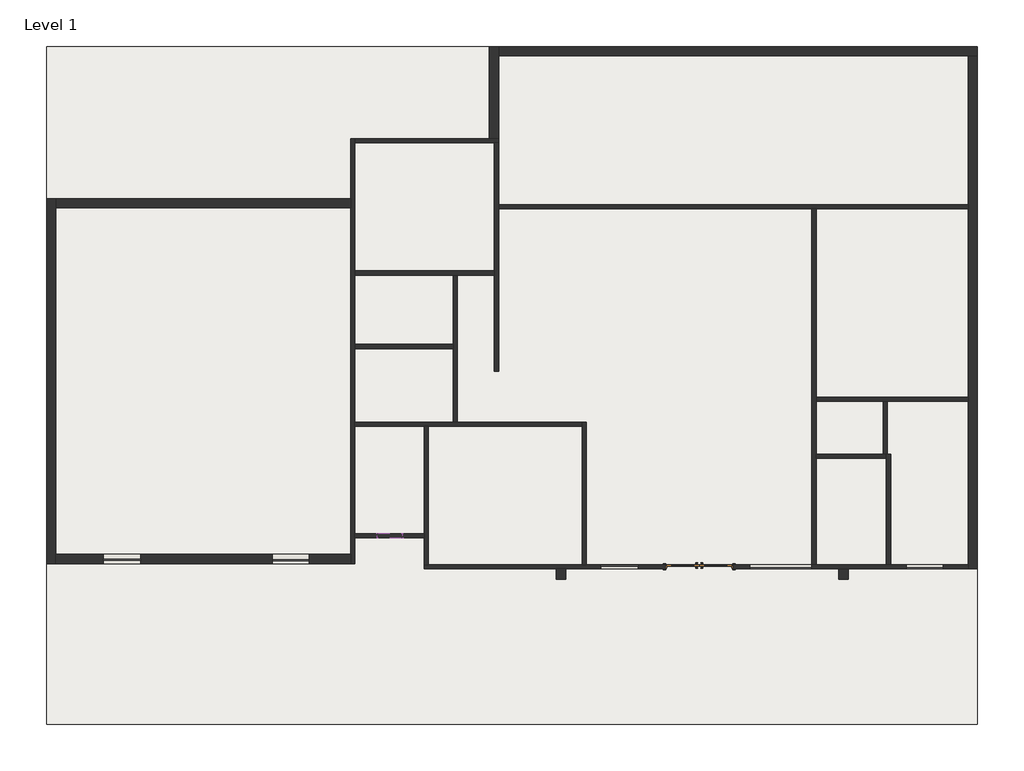
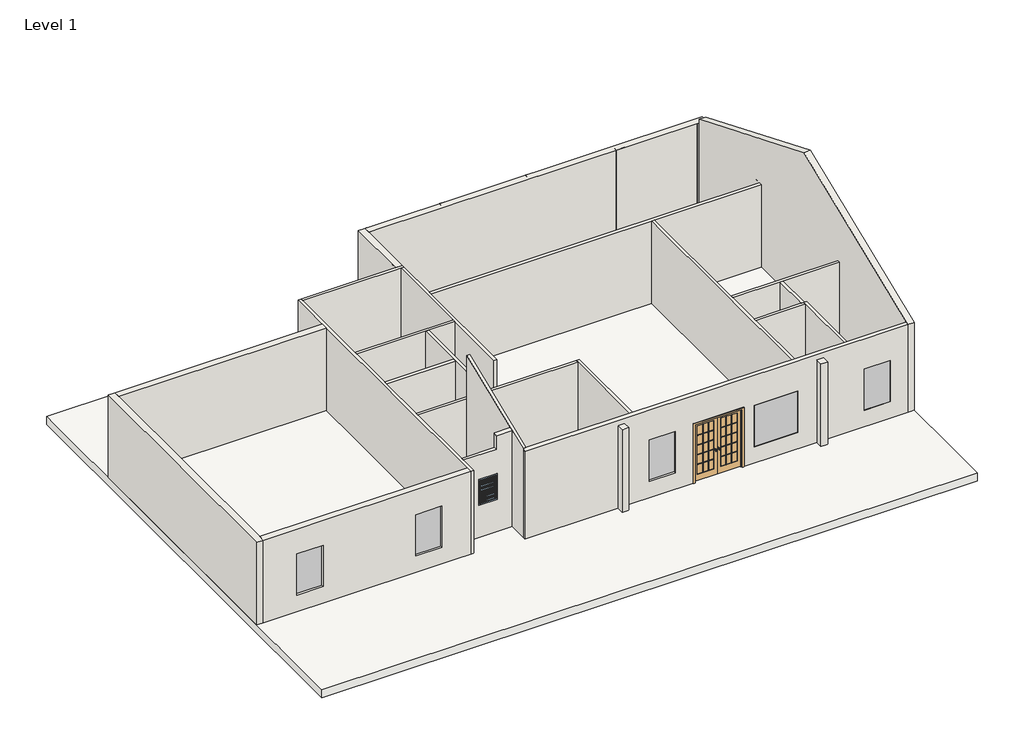
# One storey: 25 walls, 7 columns, 5 plates, 1 door, 1 slab, 1 window.
"""IFC4 building model written with IfcOpenShell, lengths in millimetres."""

from ifc_helpers import new_model, si_unit, frame, origin, origin_with_axes, place, context, project, spatial, polyline, outline, extrude, faceted_brep, transform, mapped, element, save
from components import door_09c896ac, system_panel_glazed_cdc09dc4, system_panel_glazed_afe70ed6, window_d9a389d2

model = new_model("IFC4")

# Units and contexts
model_context = context("Model", 3, world=origin())
ifc_project = project(units=[si_unit("LENGTHUNIT", "METRE", prefix="MILLI")], contexts=[model_context])

# Site, building, storey
site = spatial("IfcSite", under=ifc_project)
building = spatial("IfcBuilding", under=site)
storey = spatial("IfcBuildingStorey", under=building, Name="Level 1", Elevation=0.0)

# Columns
placement = place(None, origin())
element("IfcColumn", 1, ObjectType="Rectangular Column : 9\" x 12\"", at=placement, inside=storey, context=model_context, shape_type="SweptSolid", body=[
    extrude(outline(polyline([(-2253.6765363, 15600.9899709), (-2253.6765363, 15372.3899709), (-2329.8765363, 15372.3899709), (-2329.8765363, 15600.9899709), (-2253.6765363, 15600.9899709)])), origin_with_axes(), (0.0, 0.0, 1.0), 3048.0),
])
element("IfcColumn", 2, ObjectType="Rectangular Column : 9\" x 12\"", at=placement, inside=storey, context=model_context, shape_type="Brep", body=[
    faceted_brep([(9430.3234637, 15600.9899709, 0.0), (9430.3234637, 15372.3899709, 0.0), (9201.7234637, 15372.3899709, 0.0), (9125.5234637, 15372.3899709, 0.0), (9125.5234637, 15600.9899709, 0.0), (9430.3234637, 15600.9899709, 3048.0), (9430.3234637, 15372.3899709, 3048.0), (9125.5234637, 15372.3899709, 3048.0), (9125.5234637, 15600.9899709, 3048.0)], [[[0, 1, 2, 3, 4]], [[5, 6, 1, 0]], [[6, 7, 3, 2, 1]], [[7, 8, 4, 3]], [[8, 5, 0, 4]], [[5, 8, 7, 6]]]),
])
element("IfcColumn", 3, ObjectType="Rectangular Column : 9\" x 12\"", at=placement, inside=storey, context=model_context, shape_type="SweptSolid", body=[
    extrude(outline(polyline([(565.7234637, 15600.9899709), (565.7234637, 15372.3899709), (260.9234637, 15372.3899709), (260.9234637, 15600.9899709), (565.7234637, 15600.9899709)])), origin_with_axes(), (0.0, 0.0, 1.0), 3048.0),
])
element("IfcColumn", 4, ObjectType="Rectangular Column : 9\" x 12\"", at=placement, inside=storey, context=model_context, shape_type="SweptSolid", body=[
    extrude(outline(polyline([(3562.9234637, 15600.9899709), (3562.9234637, 15372.3899709), (3258.1234637, 15372.3899709), (3258.1234637, 15600.9899709), (3562.9234637, 15600.9899709)])), origin_with_axes(), (0.0, 0.0, 1.0), 3048.0),
])
element("IfcColumn", 5, ObjectType="Rectangular Column : 9\" x 12\"", at=placement, inside=storey, context=model_context, shape_type="SweptSolid", body=[
    extrude(outline(polyline([(6610.9234637, 15600.9899709), (6610.9234637, 15372.3899709), (6306.1234637, 15372.3899709), (6306.1234637, 15600.9899709), (6610.9234637, 15600.9899709)])), origin_with_axes(), (0.0, 0.0, 1.0), 3048.0),
])
element("IfcColumn", 6, ObjectType="Rectangular Column : 9\" x 12\"", at=placement, inside=storey, context=model_context, shape_type="SweptSolid", body=[
    extrude(outline(polyline([(-2558.4765363, 13543.5899709), (-2329.8765363, 13543.5899709), (-2329.8765363, 13340.3899709), (-2558.4765363, 13340.3899709), (-2558.4765363, 13543.5899709)])), origin_with_axes(), (0.0, 0.0, 1.0), 3048.0),
])
element("IfcColumn", 7, ObjectType="Rectangular Column : 9\" x 12\"", at=placement, inside=storey, context=model_context, shape_type="Brep", body=[
    faceted_brep([(9201.7234637, 11917.9899709, 0.0), (9430.3234637, 11917.9899709, 0.0), (9430.3234637, 11613.1899709, 0.0), (9201.7234637, 11613.1899709, 0.0), (9201.7234637, 11714.7899709, 0.0), (9201.7234637, 11917.9899709, 3048.0), (9430.3234637, 11917.9899709, 3048.0), (9430.3234637, 11613.1899709, 3048.0), (9201.7234637, 11613.1899709, 3048.0), (9201.7234637, 11714.7899709, 3048.0)], [[[0, 1, 2, 3, 4]], [[5, 6, 1, 0]], [[6, 7, 2, 1]], [[7, 8, 3, 2]], [[8, 9, 5, 0, 4, 3]], [[5, 9, 8, 7, 6]]]),
])

# Door
door_shape = door_09c896ac(model_context)
element("IfcDoor", 8, ObjectType="Door-Interior-Double-Full Glass-Wood : 64\" x 84\"", at=placement, inside=storey, context=model_context, shape_type="MappedRepresentation", body=[
    mapped(door_shape, transform((2597.7234637, 2827.9649709, 0.0), x_axis=(1.0, 0.0, 0.0), y_axis=(0.0, 1.0, 0.0), z_axis=(0.0, 0.0, 1.0))),
])

# Plates
system_panel_glazed_shape = system_panel_glazed_cdc09dc4(model_context)
element("IfcPlate", 9, ObjectType="System Panel : Glazed", at=placement, inside=storey, context=model_context, shape_type="MappedRepresentation", body=[
    mapped(system_panel_glazed_shape, transform((641.9234637, 2824.7899709, 609.6), x_axis=(1.0, 0.0, 0.0), y_axis=(0.0, 1.0, 0.0), z_axis=(0.0, 0.0, 1.0))),
])
element("IfcPlate", 10, ObjectType="System Panel : Glazed", at=placement, inside=storey, context=model_context, shape_type="MappedRepresentation", body=[
    mapped(system_panel_glazed_shape, transform((8134.9234637, 2824.7899709, 609.6), x_axis=(-1.0, 0.0, 0.0), y_axis=(0.0, -1.0, 0.0), z_axis=(0.0, 0.0, 1.0))),
])
element("IfcPlate", 11, ObjectType="System Panel : Glazed", at=placement, inside=storey, context=model_context, shape_type="MappedRepresentation", body=[
    mapped(system_panel_glazed_shape, transform((-7435.2765363, 3015.2899709, 609.6), x_axis=(-1.0, 0.0, 0.0), y_axis=(0.0, -1.0, 0.0), z_axis=(0.0, 0.0, 1.0))),
])
element("IfcPlate", 12, ObjectType="System Panel : Glazed", at=placement, inside=storey, context=model_context, shape_type="MappedRepresentation", body=[
    mapped(system_panel_glazed_shape, transform((-11575.4765363, 2964.4899709, 609.6), x_axis=(1.0, 0.0, 0.0), y_axis=(0.0, 1.0, 0.0), z_axis=(0.0, 0.0, 1.0))),
])
system_panel_glazed_2_shape = system_panel_glazed_afe70ed6(model_context)
element("IfcPlate", 13, ObjectType="System Panel : Glazed", at=placement, inside=storey, context=model_context, shape_type="MappedRepresentation", body=[
    mapped(system_panel_glazed_2_shape, transform((4604.3234637, 2824.7899709, 609.6), x_axis=(-1.0, 0.0, 0.0), y_axis=(0.0, -1.0, 0.0), z_axis=(0.0, 0.0, 1.0))),
])

# Slab
element("IfcSlab", 14, ObjectType="Generic - 12\"", at=placement, inside=storey, context=model_context, shape_type="SweptSolid", body=[
    extrude(outline(polyline([(-13429.6765363, 15600.9899709), (9430.3234637, 15600.9899709), (9430.3234637, -1037.5706845), (-13429.6765363, -1037.5706845), (-13429.6765363, 15600.9899709)])), frame((0.0, 0.0, -304.8), z_axis=(0.0, 0.0, 1.0), x_axis=(1.0, 0.0, 0.0)), (0.0, 0.0, 1.0), 304.8),
])

# Walls
element("IfcWall", 15, ObjectType="4\" wall", at=placement, inside=storey, context=model_context, shape_type="Brep", body=[
    faceted_brep([(-2329.8765363, 11613.1899709, 0.0), (5366.3234637, 11613.1899709, 0.0), (5467.9234637, 11613.1899709, 0.0), (9201.7234637, 11613.1899709, 0.0), (9201.7234637, 11613.1899709, 3048.0), (5467.9234637, 11613.1899709, 3048.0), (5366.3234637, 11613.1899709, 3048.0), (-2329.8765363, 11613.1899709, 3048.0), (-2329.8765363, 11714.7899709, 0.0), (-2329.8765363, 11714.7899709, 3048.0), (9201.7234637, 11714.7899709, 3048.0), (9201.7234637, 11714.7899709, 0.0)], [[[0, 1, 2, 3, 4, 5, 6, 7]], [[8, 9, 10, 11]], [[3, 2, 1, 0, 8, 11]], [[7, 6, 5, 4, 10, 9]], [[4, 3, 11, 10]], [[0, 7, 9, 8]]]),
])
element("IfcWall", 16, ObjectType="4\" wall", at=placement, inside=storey, context=model_context, shape_type="Brep", body=[
    faceted_brep([(5366.3234637, 11613.1899709, 0.0), (5366.3234637, 2875.5899709, 0.0), (5366.3234637, 2875.5899709, 609.6), (5366.3234637, 2875.5899709, 2133.6), (5366.3234637, 2875.5899709, 3048.0), (5366.3234637, 11613.1899709, 3048.0), (5467.9234637, 11613.1899709, 0.0), (5467.9234637, 11613.1899709, 3048.0), (5467.9234637, 6990.3899709, 3048.0), (5467.9234637, 6888.7899709, 3048.0), (5467.9234637, 5593.3899709, 3048.0), (5467.9234637, 5491.7899709, 3048.0), (5467.9234637, 2875.5899709, 3048.0), (5467.9234637, 2875.5899709, 0.0), (5467.9234637, 5491.7899709, 0.0), (5467.9234637, 5593.3899709, 0.0), (5467.9234637, 6888.7899709, 0.0), (5467.9234637, 6990.3899709, 0.0)], [[[0, 1, 2, 3, 4, 5]], [[6, 7, 8, 9, 10, 11, 12, 13, 14, 15, 16, 17]], [[1, 0, 6, 17, 16, 15, 14, 13]], [[5, 4, 12, 11, 10, 9, 8, 7]], [[0, 5, 7, 6]], [[4, 3, 2, 1, 13, 12]]]),
])
element("IfcWall", 17, ObjectType="4\" wall", at=placement, inside=storey, context=model_context, shape_type="Brep", body=[
    faceted_brep([(5467.9234637, 6888.7899709, 0.0), (7118.9234637, 6888.7899709, 0.0), (7220.5234637, 6888.7899709, 0.0), (9201.7234637, 6888.7899709, 0.0), (9201.7234637, 6888.7899709, 3048.0), (7220.5234637, 6888.7899709, 3048.0), (7118.9234637, 6888.7899709, 3048.0), (5467.9234637, 6888.7899709, 3048.0), (5467.9234637, 6990.3899709, 0.0), (5467.9234637, 6990.3899709, 3048.0), (9201.7234637, 6990.3899709, 3048.0), (9201.7234637, 6990.3899709, 0.0)], [[[0, 1, 2, 3, 4, 5, 6, 7]], [[8, 9, 10, 11]], [[3, 2, 1, 0, 8, 11]], [[7, 6, 5, 4, 10, 9]], [[4, 3, 11, 10]], [[0, 7, 9, 8]]]),
])
element("IfcWall", 18, ObjectType="4\" wall", at=placement, inside=storey, context=model_context, shape_type="Brep", body=[
    faceted_brep([(9201.7234637, 2875.5899709, 3280.369501), (9201.7234637, 2875.5899709, 0.0), (7296.7234637, 2875.5899709, 0.0), (7195.1234637, 2875.5899709, 0.0), (5467.9234637, 2875.5899709, 0.0), (5366.3234637, 2875.5899709, 0.0), (3435.9234637, 2875.5899709, 0.0), (3435.9234637, 2875.5899709, 2159.0), (1759.5234637, 2875.5899709, 2159.0), (1759.5234637, 2875.5899709, 0.0), (-170.8765363, 2875.5899709, 0.0), (-272.4765363, 2875.5899709, 0.0), (-4057.0765363, 2875.5899709, 0.0), (-4158.6765363, 2875.5899709, 0.0), (-4158.6765363, 2875.5899709, 3280.369501), (-4057.0765363, 2875.5899709, 3280.369501), (184.7234637, 2875.5899709, 2133.6), (184.7234637, 2875.5899709, 609.6), (1099.1234637, 2875.5899709, 609.6), (1099.1234637, 2875.5899709, 2133.6), (5366.3234637, 2875.5899709, 609.6), (5366.3234637, 2875.5899709, 2133.6), (3842.3234637, 2875.5899709, 2133.6), (3842.3234637, 2875.5899709, 609.6), (8592.1234637, 2875.5899709, 609.6), (8592.1234637, 2875.5899709, 2133.6), (7677.7234637, 2875.5899709, 2133.6), (7677.7234637, 2875.5899709, 609.6), (9201.7234637, 2773.9899709, 0.0), (9201.7234637, 2773.9899709, 3239.3204365), (-4158.6765363, 2773.9899709, 3239.3204365), (-4158.6765363, 2773.9899709, 0.0), (-907.4765363, 2773.9899709, 0.0), (-678.8765363, 2773.9899709, 0.0), (1759.5234637, 2773.9899709, 0.0), (1759.5234637, 2773.9899709, 2159.0), (3435.9234637, 2773.9899709, 2159.0), (3435.9234637, 2773.9899709, 0.0), (6026.7234637, 2773.9899709, 0.0), (6255.3234637, 2773.9899709, 0.0), (184.7234637, 2773.9899709, 609.6), (184.7234637, 2773.9899709, 2133.6), (1099.1234637, 2773.9899709, 2133.6), (1099.1234637, 2773.9899709, 609.6), (5366.3234637, 2773.9899709, 2133.6), (5366.3234637, 2773.9899709, 609.6), (3842.3234637, 2773.9899709, 609.6), (3842.3234637, 2773.9899709, 2133.6), (8592.1234637, 2773.9899709, 2133.6), (8592.1234637, 2773.9899709, 609.6), (7677.7234637, 2773.9899709, 609.6), (7677.7234637, 2773.9899709, 2133.6)], [[[0, 1, 2, 3, 4, 5, 6, 7, 8, 9, 10, 11, 12, 13, 14, 15], [16, 17, 18, 19], [20, 21, 22, 23], [24, 25, 26, 27]], [[28, 29, 30, 31, 32, 33, 34, 35, 36, 37, 38, 39], [40, 41, 42, 43], [44, 45, 46, 47], [48, 49, 50, 51]], [[1, 28, 39, 38, 37, 6, 5, 4, 3, 2]], [[31, 13, 12, 11, 10, 9, 34, 33, 32]], [[1, 0, 29, 28]], [[14, 13, 31, 30]], [[36, 7, 6, 37]], [[7, 36, 35, 8]], [[8, 35, 34, 9]], [[16, 41, 40, 17]], [[41, 16, 19, 42]], [[42, 19, 18, 43]], [[17, 40, 43, 18]], [[20, 45, 44, 21]], [[21, 44, 47, 22]], [[22, 47, 46, 23]], [[45, 20, 23, 46]], [[24, 49, 48, 25]], [[25, 48, 51, 26]], [[26, 51, 50, 27]], [[49, 24, 27, 50]], [[0, 15, 14, 30, 29]]]),
])
element("IfcWall", 19, ObjectType="4\" wall", at=placement, inside=storey, context=model_context, shape_type="Brep", body=[
    faceted_brep([(-170.8765363, 2875.5899709, 0.0), (-170.8765363, 6380.7899709, 0.0), (-170.8765363, 6380.7899709, 3048.0), (-170.8765363, 2875.5899709, 3048.0), (-272.4765363, 2875.5899709, 0.0), (-272.4765363, 2875.5899709, 3048.0), (-272.4765363, 6279.1899709, 3048.0), (-272.4765363, 6380.7899709, 3048.0), (-272.4765363, 6380.7899709, 0.0), (-272.4765363, 6279.1899709, 0.0)], [[[0, 1, 2, 3]], [[4, 5, 6, 7, 8, 9]], [[1, 0, 4, 9, 8]], [[3, 2, 7, 6, 5]], [[0, 3, 5, 4]], [[2, 1, 8, 7]]]),
])
element("IfcWall", 20, ObjectType="4\" wall", at=placement, inside=storey, context=model_context, shape_type="Brep", body=[
    faceted_brep([(-5860.4765363, 6279.1899709, 0.0), (-4158.6765363, 6279.1899709, 0.0), (-4057.0765363, 6279.1899709, 0.0), (-272.4765363, 6279.1899709, 0.0), (-272.4765363, 6279.1899709, 3048.0), (-5860.4765363, 6279.1899709, 3048.0), (-5860.4765363, 6380.7899709, 0.0), (-5860.4765363, 6380.7899709, 3048.0), (-3447.4765363, 6380.7899709, 3048.0), (-3345.8765363, 6380.7899709, 3048.0), (-272.4765363, 6380.7899709, 3048.0), (-272.4765363, 6380.7899709, 0.0), (-3345.8765363, 6380.7899709, 0.0), (-3447.4765363, 6380.7899709, 0.0)], [[[0, 1, 2, 3, 4, 5]], [[6, 7, 8, 9, 10, 11, 12, 13]], [[3, 2, 1, 0, 6, 13, 12, 11]], [[5, 4, 10, 9, 8, 7]], [[0, 5, 7, 6]], [[4, 3, 11, 10]]]),
])
element("IfcWall", 21, ObjectType="4\" wall", at=placement, inside=storey, context=model_context, shape_type="Brep", body=[
    faceted_brep([(-5962.0765363, 13340.3899709, 0.0), (-5962.0765363, 11867.1899709, 0.0), (-5962.0765363, 11638.5899709, 0.0), (-5962.0765363, 3129.5899709, 0.0), (-5962.0765363, 2900.9899709, 0.0), (-5962.0765363, 2900.9899709, 3048.0), (-5962.0765363, 3129.5899709, 3048.0), (-5962.0765363, 11638.5899709, 3048.0), (-5962.0765363, 11867.1899709, 3048.0), (-5962.0765363, 13340.3899709, 3048.0), (-5860.4765363, 13340.3899709, 0.0), (-5860.4765363, 13340.3899709, 3048.0), (-5860.4765363, 13238.7899709, 3048.0), (-5860.4765363, 10089.1899709, 3048.0), (-5860.4765363, 9987.5899709, 3048.0), (-5860.4765363, 8285.7899709, 3048.0), (-5860.4765363, 8184.1899709, 3048.0), (-5860.4765363, 6380.7899709, 3048.0), (-5860.4765363, 6279.1899709, 3048.0), (-5860.4765363, 3637.5899709, 3048.0), (-5860.4765363, 3535.9899709, 3048.0), (-5860.4765363, 2900.9899709, 3048.0), (-5860.4765363, 2900.9899709, 0.0), (-5860.4765363, 3535.9899709, 0.0), (-5860.4765363, 3637.5899709, 0.0), (-5860.4765363, 6279.1899709, 0.0), (-5860.4765363, 6380.7899709, 0.0), (-5860.4765363, 8184.1899709, 0.0), (-5860.4765363, 8285.7899709, 0.0), (-5860.4765363, 9987.5899709, 0.0), (-5860.4765363, 10089.1899709, 0.0), (-5860.4765363, 13238.7899709, 0.0)], [[[0, 1, 2, 3, 4, 5, 6, 7, 8, 9]], [[10, 11, 12, 13, 14, 15, 16, 17, 18, 19, 20, 21, 22, 23, 24, 25, 26, 27, 28, 29, 30, 31]], [[4, 3, 2, 1, 0, 10, 31, 30, 29, 28, 27, 26, 25, 24, 23, 22]], [[9, 8, 7, 6, 5, 21, 20, 19, 18, 17, 16, 15, 14, 13, 12, 11]], [[5, 4, 22, 21]], [[0, 9, 11, 10]]]),
])
element("IfcWall", 22, ObjectType="4\" wall", at=placement, inside=storey, context=model_context, shape_type="Brep", body=[
    faceted_brep([(-4057.0765363, 2875.5899709, 0.0), (-4057.0765363, 6279.1899709, 0.0), (-4057.0765363, 6279.1899709, 4655.5131633), (-4057.0765363, 2875.5899709, 3280.369501), (-4158.6765363, 2875.5899709, 0.0), (-4158.6765363, 2875.5899709, 3280.369501), (-4158.6765363, 3535.9899709, 3547.1884206), (-4158.6765363, 3637.5899709, 3588.2374851), (-4158.6765363, 6279.1899709, 4655.5131633), (-4158.6765363, 6279.1899709, 0.0), (-4158.6765363, 3637.5899709, 0.0), (-4158.6765363, 3535.9899709, 0.0)], [[[0, 1, 2, 3]], [[4, 5, 6, 7, 8, 9, 10, 11]], [[1, 0, 4, 11, 10, 9]], [[0, 3, 5, 4]], [[2, 1, 9, 8]], [[3, 2, 8, 7, 6, 5]]]),
])
element("IfcWall", 23, ObjectType="4\" wall", at=placement, inside=storey, context=model_context, shape_type="Brep", body=[
    faceted_brep([(-5860.4765363, 3535.9899709, 0.0), (-4158.6765363, 3535.9899709, 0.0), (-4158.6765363, 3535.9899709, 3547.1884206), (-4714.3015363, 3535.9899709, 3547.1884206), (-4714.3015363, 3535.9899709, 3048.0), (-5860.4765363, 3535.9899709, 3048.0), (-5304.8515363, 3535.9899709, 2133.6), (-4695.2515363, 3535.9899709, 2133.6), (-4695.2515363, 3535.9899709, 1219.2), (-5304.8515363, 3535.9899709, 1219.2), (-5860.4765363, 3637.5899709, 0.0), (-5860.4765363, 3637.5899709, 3048.0), (-4714.3015363, 3637.5899709, 3048.0), (-4714.3015363, 3637.5899709, 3588.2374851), (-4158.6765363, 3637.5899709, 3588.2374851), (-4158.6765363, 3637.5899709, 0.0), (-5304.8515363, 3637.5899709, 2133.6), (-5304.8515363, 3637.5899709, 1219.2), (-4695.2515363, 3637.5899709, 1219.2), (-4695.2515363, 3637.5899709, 2133.6)], [[[0, 1, 2, 3, 4, 5], [6, 7, 8, 9]], [[10, 11, 12, 13, 14, 15], [16, 17, 18, 19]], [[1, 0, 10, 15]], [[0, 5, 11, 10]], [[2, 1, 15, 14]], [[17, 16, 6, 9]], [[18, 17, 9, 8]], [[19, 18, 8, 7]], [[16, 19, 7, 6]], [[5, 4, 12, 11]], [[12, 4, 3, 13]], [[3, 2, 14, 13]]]),
])
element("IfcWall", 24, ObjectType="4\" wall", at=placement, inside=storey, context=model_context, shape_type="Brep", body=[
    faceted_brep([(-5860.4765363, 9987.5899709, 0.0), (-3447.4765363, 9987.5899709, 0.0), (-3345.8765363, 9987.5899709, 0.0), (-2431.4765363, 9987.5899709, 0.0), (-2431.4765363, 9987.5899709, 3048.0), (-3345.8765363, 9987.5899709, 3048.0), (-3447.4765363, 9987.5899709, 3048.0), (-5860.4765363, 9987.5899709, 3048.0), (-5860.4765363, 10089.1899709, 0.0), (-5860.4765363, 10089.1899709, 3048.0), (-2431.4765363, 10089.1899709, 3048.0), (-2431.4765363, 10089.1899709, 0.0)], [[[0, 1, 2, 3, 4, 5, 6, 7]], [[8, 9, 10, 11]], [[3, 2, 1, 0, 8, 11]], [[7, 6, 5, 4, 10, 9]], [[4, 3, 11, 10]], [[0, 7, 9, 8]]]),
])
element("IfcWall", 25, ObjectType="4\" wall", at=placement, inside=storey, context=model_context, shape_type="Brep", body=[
    faceted_brep([(-5860.4765363, 13238.7899709, 0.0), (-2431.4765363, 13238.7899709, 0.0), (-2329.8765363, 13238.7899709, 0.0), (-2329.8765363, 13238.7899709, 3048.0), (-2431.4765363, 13238.7899709, 3048.0), (-5860.4765363, 13238.7899709, 3048.0), (-5860.4765363, 13340.3899709, 0.0), (-5860.4765363, 13340.3899709, 3048.0), (-2558.4765363, 13340.3899709, 3048.0), (-2329.8765363, 13340.3899709, 3048.0), (-2329.8765363, 13340.3899709, 0.0), (-2558.4765363, 13340.3899709, 0.0)], [[[0, 1, 2, 3, 4, 5]], [[6, 7, 8, 9, 10, 11]], [[2, 1, 0, 6, 11, 10]], [[5, 4, 3, 9, 8, 7]], [[0, 5, 7, 6]], [[3, 2, 10, 9]]]),
])
element("IfcWall", 26, ObjectType="4\" wall", at=placement, inside=storey, context=model_context, shape_type="Brep", body=[
    faceted_brep([(-3447.4765363, 9987.5899709, 0.0), (-3447.4765363, 8285.7899709, 0.0), (-3447.4765363, 8184.1899709, 0.0), (-3447.4765363, 6380.7899709, 0.0), (-3447.4765363, 6380.7899709, 3048.0), (-3447.4765363, 8184.1899709, 3048.0), (-3447.4765363, 8285.7899709, 3048.0), (-3447.4765363, 9987.5899709, 3048.0), (-3345.8765363, 9987.5899709, 0.0), (-3345.8765363, 9987.5899709, 3048.0), (-3345.8765363, 6380.7899709, 3048.0), (-3345.8765363, 6380.7899709, 0.0)], [[[0, 1, 2, 3, 4, 5, 6, 7]], [[8, 9, 10, 11]], [[3, 2, 1, 0, 8, 11]], [[7, 6, 5, 4, 10, 9]], [[4, 3, 11, 10]], [[0, 7, 9, 8]]]),
])
element("IfcWall", 27, ObjectType="4\" wall", at=placement, inside=storey, context=model_context, shape_type="SweptSolid", body=[
    extrude(outline(polyline([(-5860.4765363, 8285.7899709), (-3447.4765363, 8285.7899709), (-3447.4765363, 8184.1899709), (-5860.4765363, 8184.1899709), (-5860.4765363, 8285.7899709)])), origin_with_axes(), (0.0, 0.0, 1.0), 3048.0),
])
element("IfcWall", 28, ObjectType="4\" wall", at=placement, inside=storey, context=model_context, shape_type="Brep", body=[
    faceted_brep([(7296.7234637, 2875.5899709, 0.0), (7296.7234637, 5593.3899709, 0.0), (7296.7234637, 5593.3899709, 3048.0), (7296.7234637, 2875.5899709, 3048.0), (7195.1234637, 2875.5899709, 0.0), (7195.1234637, 2875.5899709, 3048.0), (7195.1234637, 5491.7899709, 3048.0), (7195.1234637, 5593.3899709, 3048.0), (7195.1234637, 5593.3899709, 0.0), (7195.1234637, 5491.7899709, 0.0), (7220.5234637, 5593.3899709, 0.0), (7220.5234637, 5593.3899709, 3048.0)], [[[0, 1, 2, 3]], [[4, 5, 6, 7, 8, 9]], [[1, 0, 4, 9, 8, 10]], [[3, 2, 11, 7, 6, 5]], [[0, 3, 5, 4]], [[2, 1, 10, 8, 7, 11]]]),
])
element("IfcWall", 29, ObjectType="4\" wall", at=placement, inside=storey, context=model_context, shape_type="Brep", body=[
    faceted_brep([(5467.9234637, 5491.7899709, 0.0), (7195.1234637, 5491.7899709, 0.0), (7195.1234637, 5491.7899709, 3048.0), (5467.9234637, 5491.7899709, 3048.0), (5467.9234637, 5593.3899709, 0.0), (5467.9234637, 5593.3899709, 3048.0), (7118.9234637, 5593.3899709, 3048.0), (7195.1234637, 5593.3899709, 3048.0), (7195.1234637, 5593.3899709, 0.0), (7118.9234637, 5593.3899709, 0.0)], [[[0, 1, 2, 3]], [[4, 5, 6, 7, 8, 9]], [[1, 0, 4, 9, 8]], [[3, 2, 7, 6, 5]], [[0, 3, 5, 4]], [[2, 1, 8, 7]]]),
])
element("IfcWall", 30, ObjectType="4\" wall", at=placement, inside=storey, context=model_context, shape_type="Brep", body=[
    faceted_brep([(7118.9234637, 6888.7899709, 0.0), (7118.9234637, 5593.3899709, 0.0), (7118.9234637, 5593.3899709, 3048.0), (7118.9234637, 6888.7899709, 3048.0), (7220.5234637, 6888.7899709, 0.0), (7220.5234637, 6888.7899709, 3048.0), (7220.5234637, 5593.3899709, 3048.0), (7220.5234637, 5593.3899709, 0.0), (7195.1234637, 5593.3899709, 0.0), (7195.1234637, 5593.3899709, 3048.0)], [[[0, 1, 2, 3]], [[4, 5, 6, 7]], [[1, 0, 4, 7, 8]], [[3, 2, 9, 6, 5]], [[0, 3, 5, 4]], [[2, 1, 8, 7, 6, 9]]]),
])
element("IfcWall", 31, ObjectType="4\" wall", at=placement, inside=storey, context=model_context, shape_type="Brep", body=[
    faceted_brep([(-2431.4765363, 13238.7899709, 0.0), (-2431.4765363, 10089.1899709, 0.0), (-2431.4765363, 9987.5899709, 0.0), (-2431.4765363, 7625.3899709, 0.0), (-2431.4765363, 7625.3899709, 3048.0), (-2431.4765363, 9987.5899709, 3048.0), (-2431.4765363, 10089.1899709, 3048.0), (-2431.4765363, 13238.7899709, 3048.0), (-2329.8765363, 13238.7899709, 0.0), (-2329.8765363, 13238.7899709, 3048.0), (-2329.8765363, 11714.7899709, 3048.0), (-2329.8765363, 11613.1899709, 3048.0), (-2329.8765363, 7625.3899709, 3048.0), (-2329.8765363, 7625.3899709, 0.0), (-2329.8765363, 11613.1899709, 0.0), (-2329.8765363, 11714.7899709, 0.0)], [[[0, 1, 2, 3, 4, 5, 6, 7]], [[8, 9, 10, 11, 12, 13, 14, 15]], [[3, 2, 1, 0, 8, 15, 14, 13]], [[4, 3, 13, 12]], [[7, 6, 5, 4, 12, 11, 10, 9]], [[0, 7, 9, 8]]]),
])
element("IfcWall", 32, ObjectType="9\" wall", at=placement, inside=storey, context=model_context, shape_type="Brep", body=[
    faceted_brep([(9201.7234637, 15372.3899709, 0.0), (9201.7234637, 11714.7899709, 0.0), (9201.7234637, 11613.1899709, 0.0), (9201.7234637, 6990.3899709, 0.0), (9201.7234637, 6888.7899709, 0.0), (9201.7234637, 2875.5899709, 0.0), (9201.7234637, 2773.9899709, 0.0), (9201.7234637, 2773.9899709, 3239.3204365), (9201.7234637, 2875.5899709, 3280.369501), (9201.7234637, 9059.8538949, 5778.9743138), (9201.7234637, 15372.3899709, 3171.6224564), (9430.3234637, 15372.3899709, 0.0), (9430.3234637, 15372.3899709, 3048.0), (9430.3234637, 15372.3899709, 3171.6224564), (9430.3234637, 9059.8538949, 5778.9743138), (9430.3234637, 2773.9899709, 3239.3204365), (9430.3234637, 2773.9899709, 0.0)], [[[0, 1, 2, 3, 4, 5, 6, 7, 8, 9, 10]], [[11, 12, 13, 14, 15, 16]], [[6, 5, 4, 3, 2, 1, 0, 11, 16]], [[0, 10, 13, 12, 11]], [[7, 6, 16, 15]], [[10, 9, 14, 13]], [[9, 8, 7, 15, 14]]]),
])
element("IfcWall", 33, ObjectType="9\" wall", at=placement, inside=storey, context=model_context, shape_type="Brep", body=[
    faceted_brep([(-2558.4765363, 15600.9899709, 0.0), (-2558.4765363, 13340.3899709, 0.0), (-2558.4765363, 13340.3899709, 3048.0), (-2558.4765363, 15600.9899709, 3048.0), (-2329.8765363, 15600.9899709, 0.0), (-2329.8765363, 15600.9899709, 3048.0), (-2329.8765363, 15372.3899709, 3048.0), (-2329.8765363, 13340.3899709, 3048.0), (-2329.8765363, 13340.3899709, 0.0), (-2329.8765363, 15372.3899709, 0.0)], [[[0, 1, 2, 3]], [[4, 5, 6, 7, 8, 9]], [[1, 0, 4, 9, 8]], [[3, 2, 7, 6, 5]], [[0, 3, 5, 4]], [[2, 1, 8, 7]]]),
])
element("IfcWall", 34, ObjectType="9\" wall", at=placement, inside=storey, context=model_context, shape_type="Brep", body=[
    faceted_brep([(-13429.6765363, 11867.1899709, 0.0), (-13429.6765363, 2900.9899709, 0.0), (-13429.6765363, 2900.9899709, 3048.0), (-13429.6765363, 11867.1899709, 3048.0), (-13201.0765363, 11867.1899709, 0.0), (-13201.0765363, 11867.1899709, 3048.0), (-13201.0765363, 11638.5899709, 3048.0), (-13201.0765363, 3129.5899709, 3048.0), (-13201.0765363, 2900.9899709, 3048.0), (-13201.0765363, 2900.9899709, 0.0), (-13201.0765363, 3129.5899709, 0.0), (-13201.0765363, 11638.5899709, 0.0)], [[[0, 1, 2, 3]], [[4, 5, 6, 7, 8, 9, 10, 11]], [[1, 0, 4, 11, 10, 9]], [[3, 2, 8, 7, 6, 5]], [[2, 1, 9, 8]], [[0, 3, 5, 4]]]),
])
element("IfcWall", 35, ObjectType="9\" wall", at=placement, inside=storey, context=model_context, shape_type="SweptSolid", body=[
    extrude(outline(polyline([(-678.8765363, 2773.9899709), (-678.8765363, 2519.9899709), (-907.4765363, 2519.9899709), (-907.4765363, 2773.9899709), (-678.8765363, 2773.9899709)])), origin_with_axes(), (0.0, 0.0, 1.0), 3048.0),
])
element("IfcWall", 36, ObjectType="9\" wall", at=placement, inside=storey, context=model_context, shape_type="SweptSolid", body=[
    extrude(outline(polyline([(6026.7234637, 2519.9899709), (6026.7234637, 2773.9899709), (6255.3234637, 2773.9899709), (6255.3234637, 2519.9899709), (6026.7234637, 2519.9899709)])), origin_with_axes(), (0.0, 0.0, 1.0), 3048.0),
])
element("IfcWall", 37, ObjectType="9\" wall", at=placement, inside=storey, context=model_context, shape_type="SweptSolid", body=[
    extrude(outline(polyline([(0.0, -13201.0765363), (0.0, -5962.0765363), (3048.0, -5962.0765363), (3048.0, -13201.0765363), (0.0, -13201.0765363)]), holes=[polyline([(609.6, -12032.6765363), (2133.6, -12032.6765363), (2133.6, -11118.2765363), (609.6, -11118.2765363), (609.6, -12032.6765363)]), polyline([(2133.6, -6978.0765363), (609.6, -6978.0765363), (609.6, -7892.4765363), (2133.6, -7892.4765363), (2133.6, -6978.0765363)])]), frame((0.0, 2900.9899709, 0.0), z_axis=(0.0, 1.0, 0.0), x_axis=(0.0, 0.0, 1.0)), (0.0, 0.0, 1.0), 228.6),
])
element("IfcWall", 38, ObjectType="9\" wall", at=placement, inside=storey, context=model_context, shape_type="SweptSolid", body=[
    extrude(outline(polyline([(-5962.0765363, 11638.5899709), (-13201.0765363, 11638.5899709), (-13201.0765363, 11867.1899709), (-5962.0765363, 11867.1899709), (-5962.0765363, 11638.5899709)])), origin_with_axes(), (0.0, 0.0, 1.0), 3048.0),
])
element("IfcWall", 39, ObjectType="9\" wall", at=placement, inside=storey, context=model_context, shape_type="Brep", body=[
    faceted_brep([(-2329.8765363, 15372.3899709, 0.0), (9201.7234637, 15372.3899709, 0.0), (9430.3234637, 15372.3899709, 0.0), (9430.3234637, 15372.3899709, 3048.0), (-2329.8765363, 15372.3899709, 3048.0), (-2329.8765363, 15600.9899709, 0.0), (-2329.8765363, 15600.9899709, 3048.0), (9430.3234637, 15600.9899709, 3048.0), (9430.3234637, 15600.9899709, 0.0)], [[[0, 1, 2, 3, 4]], [[5, 6, 7, 8]], [[2, 1, 0, 5, 8]], [[4, 3, 7, 6]], [[3, 2, 8, 7]], [[0, 4, 6, 5]]]),
])

# Window
window_shape = window_d9a389d2(model_context)
element("IfcWindow", 40, ObjectType="Window-Louvers : 24\" x 36\"", at=placement, inside=storey, context=model_context, shape_type="MappedRepresentation", body=[
    mapped(window_shape, transform((-5000.0515363, 3593.1399709, 304.8), x_axis=(1.0, 0.0, 0.0), y_axis=(0.0, 1.0, 0.0), z_axis=(0.0, 0.0, 1.0))),
])

save(model, "model.ifc")

# Revit data of these elements
# Type "Rectangular Column : 9\" x 12\""
#   Assembly Code = "B1010200"
#   Depth = 0' - 9"
#   Offset Base = 0' - 0"
#   Offset Top = 0' - 0"
#   Width = 1' - 0"
#   Material = none
# Type "Door-Interior-Double-Full Glass-Wood : 64\" x 84\""
#   Type Mark = "8"
#   Assembly Code = "C1020300"
#   Analytic Construction = "French door, wood frame with single glass"
#   Top Rail = 0' - 4 11/16"
#   Thickness = 0' - 1 3/8"
#   Thermal Resistance (R) = 1.0696 (h·ft²·°F)/BTU
#   Swing Angle [instance default] = 90.00°
#   Stiles = 0' - 4 3/4"
#   Rough Width = 5' - 6"
#   Rough Height = 7' - 1"
#   Panel Width = 2' - 8"
#   Height = 7' - 0"
#   Width = 5' - 4"
#   Heat Transfer Coefficient (U) = 0.9350 BTU/(h·ft²·°F)
#   Bottom Rail = 0' - 9 1/8"
#   Show Grill [instance default] = yes
#   Trim Material = Cherry
#   Panel Material = Cherry
#   Frame Material = Cherry
#   Door Handle Material = Aluminum
#   Visual Light Transmittance = 0
#   Solar Heat Gain Coefficient = 0
#   Wall Closure = (empty or 0)
#   Function = (empty or 0)
# Type "System Panel : Glazed"
#   Construction Type Id = "GSP4R"
#   Analytic Construction = "1/8 in Pilkington single glazing"
#   Visual Light Transmittance = 0.9
#   Solar Heat Gain Coefficient = 0.86
#   Heat Transfer Coefficient (U) = 1.18115 BTU/(h·ft²·°F)
#   Define Thermal Properties by = 1
# Type "Generic - 12\""
#   Assembly Code = "B1010"
#   Function = 0
#   Layers, outside or top first: 1' - 0" no material (function 1)
# Type "4\" wall"
#   Assembly Code = "B2010"
#   Layers, outside or top first: 0' - 4" no material (function 1)
# Type "9\" wall"
#   Assembly Code = "B2010"
#   Layers, outside or top first: 0' - 9" no material (function 1)
# Type "Window-Louvers : 24\" x 36\""
#   Type Mark = "20"
#   Construction Type Id = "GSP4R"
#   Assembly Code = "B20"
#   Analytic Construction = "1/8 in Pilkington single glazing"
#   Visual Light Transmittance = 0.9
#   Thermal Resistance (R) = 1.53941 (h·ft²·°F)/BTU
#   Solar Heat Gain Coefficient = 0.78
#   Max Height = 3' - 0.71751"
#   Height = 3' - 0"
#   Heat Transfer Coefficient (U) = 0.6496 BTU/(h·ft²·°F)
#   Blade Width [instance default] = 1' - 10 1/2"
#   Blade Vertical Thickness = 0' - 0.35355"
#   Blade Thickness = 0' - 0 1/4"
#   Blade Spacing = 0' - 1 1/2"
#   Blade Height = 0' - 1.85355"
#   Blade Depth = 0' - 3"
#   Blade Angle = 45.00°
#   Default Sill Height = 3' - 0"
#   Trim Projection_Exterior = 0' - 0 1/2"
#   Trim Projection_Interior = 0' - 0 1/2"
#   Trim Width_Exterior = 0' - 1 1/2"
#   Trim Width_Interior = 0' - 1 1/2"
#   Width = 2' - 0"
#   Max Blade Count = 19
#   Define Thermal Properties by = 1
#   Blade Count = 18
#   Frame Material = Birch
#   Louver Material = Birch
#   Trim Exterior Material = Birch
#   Trim Interior Material = Birch
#   Wall Closure = (empty or 0)
# Elements 1, 2, 6, 7 (IfcColumn, "Rectangular Column : 9\" x 12\"")
#   Phase Created = New Construction
#   Materials on its faces: "Default Wall"
# Elements 3, 4, 5 (IfcColumn, "Rectangular Column : 9\" x 12\"")
#   Phase Created = New Construction
# Element 8 (IfcDoor, "Door-Interior-Double-Full Glass-Wood : 64\" x 84\"")
#   Swing Angle = 90.00°
#   Show Grill = yes
#   Phase Created = New Construction
#   Materials on its faces: "Cherry", "Aluminum", "Glass"
# Elements 9, 10, 11, 12, 13 (IfcPlate, "System Panel : Glazed")
#   Phase Created = New Construction
#   Materials on its faces: "Glass"
# Element 14 (IfcSlab, "Generic - 12\"")
#   built-in parameter 1001955 = 3.14159 (stored number, unit not read)
#   Height Offset From Level = 0' - 0"
#   Phase Created = New Construction
#   Materials on its faces: "Default Floor"
# Elements 15, 16, 17, 18, 19, 20, 21, 22, 23, 24, 25, 26, 27, 28, 29, 30, 31 (IfcWall, "4\" wall")
#   Top Offset = 0' - 0"
#   Base Offset = 0' - 0"
#   wall height = 10' - 0"
#   Phase Created = New Construction
#   Base Constraint = Level 1
#   Top Constraint = Level 2
#   Materials on its faces: "Default Wall"
# Elements 32, 33, 34, 35, 36, 37, 38, 39 (IfcWall, "9\" wall")
#   Top Offset = 0' - 0"
#   Base Offset = 0' - 0"
#   wall height = 10' - 0"
#   Phase Created = New Construction
#   Base Constraint = Level 1
#   Top Constraint = Level 2
#   Materials on its faces: "Default Wall"
# Element 40 (IfcWindow, "Window-Louvers : 24\" x 36\"")
#   Mark = "1"
#   Blade Width = 1' - 10 1/2"
#   Phase Created = New Construction
#   Materials on its faces: "Birch"
# Materials
#   "Cherry": class "Wood", colour RGB 226 177 128, transparency 0, Description = "Prunus Serotina", Cost = 0
#   "Aluminum": class "Metal", colour RGB 247 247 247, transparency 0, Description = "Aluminum 6061", Cost = 0
#   "Birch": class "Wood", colour RGB 224 178 126, transparency 0, Description = "Betula Alleghaniensis", Cost = 0
#   "Default Wall": colour RGB 128 128 128, transparency 0, Cost = 0
#   "Glass": class "Glass", colour RGB 0 128 192, transparency 0.75, Description = "Soda Lime Glass", Cost = 0
#   "Default Floor": colour RGB 128 128 128, transparency 0, Cost = 0
